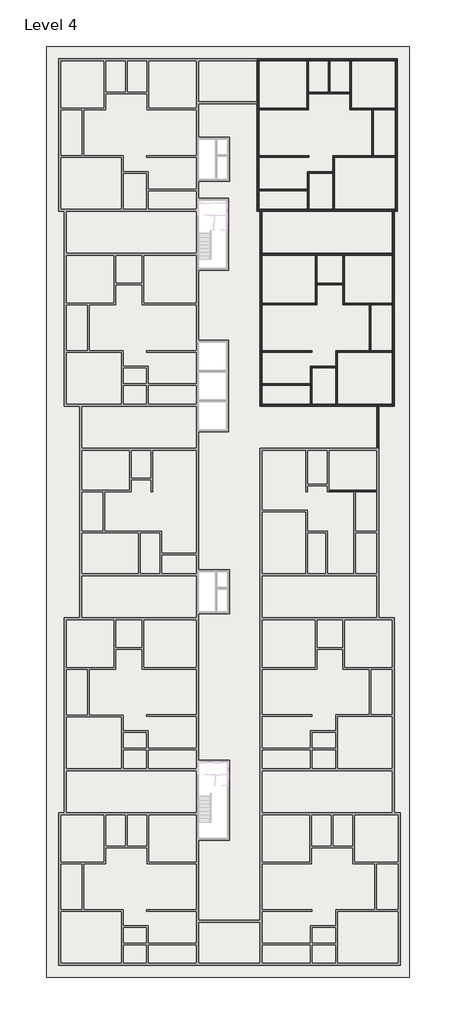
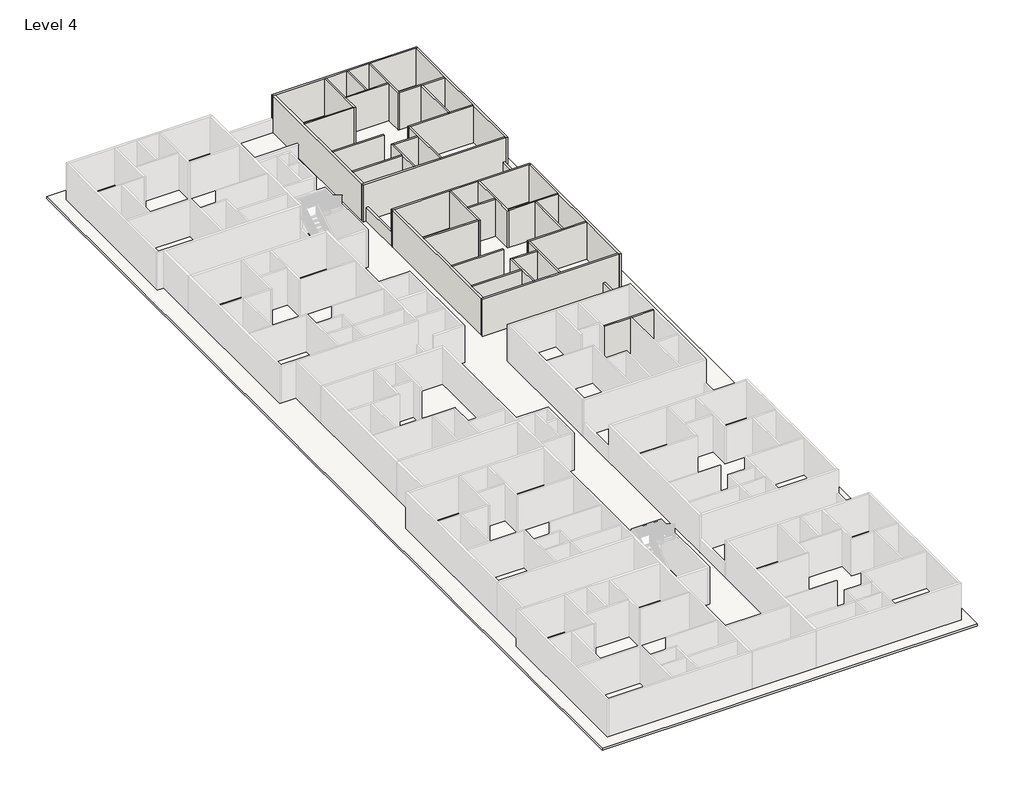
# One storey, part 4 of 8: 37 walls, 1 roof, 1 slab.
"""IFC4 building model written with IfcOpenShell, lengths in millimetres."""

from ifc_helpers import new_model, si_unit, frame, origin, place, context, project, spatial, polyline, outline, extrude, faceted_brep, element, save

model = new_model("IFC4")

# Units and contexts
model_context = context("Model", 3, world=origin())
ifc_project = project(units=[si_unit("LENGTHUNIT", "METRE", prefix="MILLI")], contexts=[model_context])

# Site, building, storey
site = spatial("IfcSite", under=ifc_project)
building = spatial("IfcBuilding", under=site)
storey = spatial("IfcBuildingStorey", under=building, Name="Level 4", Elevation=34378.6172466)

# Roof
placement = place(None, origin())
element("IfcRoof", 1, ObjectType="SLAB", at=placement, inside=storey, context=model_context, shape_type="SweptSolid", body=[
    extrude(outline(polyline([(-15237.9415084, -35021.5344126), (-15237.9415084, 36097.9216096), (12498.9443719, 36097.9216096), (12498.9443719, -35021.5344126), (-15237.9415084, -35021.5344126)]), holes=[polyline([(-3617.4415084, 29152.4900967), (-3617.4415084, 25799.6900967), (-1255.2415084, 25799.6900967), (-1255.2415084, 29152.4900967), (-3617.4415084, 29152.4900967)]), polyline([(-3617.4415084, 24490.1216096), (-3617.4415084, 19003.7216096), (-1331.4415084, 19003.7216096), (-1331.4415084, 24490.1216096), (-3617.4415084, 24490.1216096)]), polyline([(-3617.4415084, 13669.6303368), (-3617.4415084, 6659.2303368), (-1331.4415084, 6659.2303368), (-1331.4415084, 13669.6303368), (-3617.4415084, 13669.6303368)]), polyline([(-3617.4415084, -3882.2751812), (-3617.4415084, -7235.0751812), (-1255.2415084, -7235.0751812), (-1255.2415084, -3882.2751812), (-3617.4415084, -3882.2751812)]), polyline([(-3617.4415084, -18429.9851539), (-3617.4415084, -24525.9851539), (-1229.8415084, -24525.9851539), (-1229.8415084, -18429.9851539), (-3617.4415084, -18429.9851539)])]), frame((0.0, 0.0, 34378.6172466), z_axis=(0.0, 0.0, 1.0), x_axis=(1.0, 0.0, 0.0)), (0.0, 0.0, 1.0), 152.4),
])

# Slab
element("IfcSlab", 2, ObjectType="FLOOR", at=placement, inside=storey, context=model_context, shape_type="SweptSolid", body=[
    extrude(outline(polyline([(-14323.5415084, 35183.5216096), (11584.5443719, 35183.5216096), (11584.5443719, 23499.5216096), (11360.9214687, 23499.5216096), (11360.9214687, 8615.1216096), (10173.4714687, 8615.1216096), (10173.4714687, -7538.7344126), (11360.9214687, -7538.7344126), (11360.9214687, -22423.1344126), (11813.0584916, -22423.1344126), (11813.0584916, -34107.1344126), (11584.5443719, -34107.1344126), (-14323.5415084, -34107.1344126), (-14323.5415084, 35183.5216096)]), holes=[polyline([(-3617.4415084, 29152.4900967), (-3617.4415084, 25799.6900967), (-1255.2415084, 25799.6900967), (-1255.2415084, 29152.4900967), (-3617.4415084, 29152.4900967)]), polyline([(-3617.4415084, 24490.1216096), (-3617.4415084, 19003.7216096), (-1331.4415084, 19003.7216096), (-1331.4415084, 24490.1216096), (-3617.4415084, 24490.1216096)]), polyline([(-3617.4415084, 13669.6303368), (-3617.4415084, 6659.2303368), (-1331.4415084, 6659.2303368), (-1331.4415084, 13669.6303368), (-3617.4415084, 13669.6303368)]), polyline([(-3617.4415084, -3882.2751812), (-3617.4415084, -7235.0751812), (-1255.2415084, -7235.0751812), (-1255.2415084, -3882.2751812), (-3617.4415084, -3882.2751812)]), polyline([(-3617.4415084, -18429.9851539), (-3617.4415084, -24525.9851539), (-1229.8415084, -24525.9851539), (-1229.8415084, -18429.9851539), (-3617.4415084, -18429.9851539)])]), frame((0.0, 0.0, 33769.0172466), z_axis=(0.0, 0.0, 1.0), x_axis=(1.0, 0.0, 0.0)), (0.0, 0.0, 1.0), 609.6),
])

# Walls
element("IfcWall", 3, ObjectType="4.5\"", at=placement, inside=storey, context=model_context, shape_type="Brep", body=[
    faceted_brep([(6363.4714687, 2100.0216096, 34378.6172466), (8282.4584916, 2100.0216096, 34378.6172466), (8396.7584916, 2100.0216096, 34378.6172466), (10021.0714687, 2100.0216096, 34378.6172466), (10021.0714687, 2100.0216096, 37426.6172466), (8396.7584916, 2100.0216096, 37426.6172466), (8282.4584916, 2100.0216096, 37426.6172466), (6363.4714687, 2100.0216096, 37426.6172466), (6363.4714687, 2214.3216096, 34378.6172466), (6363.4714687, 2214.3216096, 37426.6172466), (10021.0714687, 2214.3216096, 37426.6172466), (10021.0714687, 2214.3216096, 34378.6172466)], [[[0, 1, 2, 3, 4, 5, 6, 7]], [[8, 9, 10, 11]], [[3, 2, 1, 0, 8, 11]], [[0, 7, 9, 8]], [[4, 3, 11, 10]], [[7, 6, 5, 4, 10, 9]]]),
])
element("IfcWall", 4, ObjectType="4.5\"", at=placement, inside=storey, context=model_context, shape_type="Brep", body=[
    faceted_brep([(5315.7214687, 20146.7216096, 34378.6172466), (5315.7214687, 16489.1216096, 34378.6172466), (5315.7214687, 16374.8216096, 34378.6172466), (5315.7214687, 16374.8216096, 37426.6172466), (5315.7214687, 16489.1216096, 37426.6172466), (5315.7214687, 20146.7216096, 37426.6172466), (5430.0214687, 20146.7216096, 34378.6172466), (5430.0214687, 20146.7216096, 37426.6172466), (5430.0214687, 18013.1216096, 37426.6172466), (5430.0214687, 17898.8216096, 37426.6172466), (5430.0214687, 16374.8216096, 37426.6172466), (5430.0214687, 16374.8216096, 34378.6172466), (5430.0214687, 17898.8216096, 34378.6172466), (5430.0214687, 18013.1216096, 34378.6172466)], [[[0, 1, 2, 3, 4, 5]], [[6, 7, 8, 9, 10, 11, 12, 13]], [[2, 1, 0, 6, 13, 12, 11]], [[0, 5, 7, 6]], [[3, 2, 11, 10]], [[5, 4, 3, 10, 9, 8, 7]]]),
])
element("IfcWall", 5, ObjectType="4.5\"", at=placement, inside=storey, context=model_context, shape_type="SweptSolid", body=[
    extrude(outline(polyline([(1259.3584916, 16489.1216096), (5315.7214687, 16489.1216096), (5315.7214687, 16374.8216096), (1259.3584916, 16374.8216096), (1259.3584916, 16489.1216096)])), frame((0.0, 0.0, 34378.6172466), z_axis=(0.0, 0.0, 1.0), x_axis=(1.0, 0.0, 0.0)), (0.0, 0.0, 1.0), 3048.0),
])
element("IfcWall", 6, ObjectType="4.5\"", at=placement, inside=storey, context=model_context, shape_type="SweptSolid", body=[
    extrude(outline(polyline([(7436.6214687, 17898.8216096), (5430.0214687, 17898.8216096), (5430.0214687, 18013.1216096), (7436.6214687, 18013.1216096), (7436.6214687, 17898.8216096)])), frame((0.0, 0.0, 34378.6172466), z_axis=(0.0, 0.0, 1.0), x_axis=(1.0, 0.0, 0.0)), (0.0, 0.0, 1.0), 3048.0),
])
element("IfcWall", 7, ObjectType="4.5\"", at=placement, inside=storey, context=model_context, shape_type="Brep", body=[
    faceted_brep([(7436.6214687, 20146.7216096, 34378.6172466), (7436.6214687, 18013.1216096, 34378.6172466), (7436.6214687, 17898.8216096, 34378.6172466), (7436.6214687, 16374.8216096, 34378.6172466), (7436.6214687, 16374.8216096, 37426.6172466), (7436.6214687, 17898.8216096, 37426.6172466), (7436.6214687, 18013.1216096, 37426.6172466), (7436.6214687, 20146.7216096, 37426.6172466), (7550.9214687, 20146.7216096, 34378.6172466), (7550.9214687, 20146.7216096, 37426.6172466), (7550.9214687, 16489.1216096, 37426.6172466), (7550.9214687, 16374.8216096, 37426.6172466), (7550.9214687, 16374.8216096, 34378.6172466), (7550.9214687, 16489.1216096, 34378.6172466)], [[[0, 1, 2, 3, 4, 5, 6, 7]], [[8, 9, 10, 11, 12, 13]], [[3, 2, 1, 0, 8, 13, 12]], [[0, 7, 9, 8]], [[4, 3, 12, 11]], [[7, 6, 5, 4, 11, 10, 9]]]),
])
element("IfcWall", 8, ObjectType="4.5\"", at=placement, inside=storey, context=model_context, shape_type="Brep", body=[
    faceted_brep([(7550.9214687, 16374.8216096, 34378.6172466), (9469.9084916, 16374.8216096, 34378.6172466), (9584.2084916, 16374.8216096, 34378.6172466), (11208.5214687, 16374.8216096, 34378.6172466), (11208.5214687, 16374.8216096, 37426.6172466), (9584.2084916, 16374.8216096, 37426.6172466), (9469.9084916, 16374.8216096, 37426.6172466), (7550.9214687, 16374.8216096, 37426.6172466), (7550.9214687, 16489.1216096, 34378.6172466), (7550.9214687, 16489.1216096, 37426.6172466), (11208.5214687, 16489.1216096, 37426.6172466), (11208.5214687, 16489.1216096, 34378.6172466)], [[[0, 1, 2, 3, 4, 5, 6, 7]], [[8, 9, 10, 11]], [[3, 2, 1, 0, 8, 11]], [[0, 7, 9, 8]], [[4, 3, 11, 10]], [[7, 6, 5, 4, 10, 9]]]),
])
element("IfcWall", 9, ObjectType="4.5\"", at=placement, inside=storey, context=model_context, shape_type="SweptSolid", body=[
    extrude(outline(polyline([(9469.9084916, 12869.6216096), (9469.9084916, 16374.8216096), (9584.2084916, 16374.8216096), (9584.2084916, 12869.6216096), (9469.9084916, 12869.6216096)])), frame((0.0, 0.0, 34378.6172466), z_axis=(0.0, 0.0, 1.0), x_axis=(1.0, 0.0, 0.0)), (0.0, 0.0, 1.0), 3048.0),
])
element("IfcWall", 10, ObjectType="4.5\"", at=placement, inside=storey, context=model_context, shape_type="Brep", body=[
    faceted_brep([(11208.5214687, 12869.6216096, 34378.6172466), (9584.2084916, 12869.6216096, 34378.6172466), (9469.9084916, 12869.6216096, 34378.6172466), (6885.4584916, 12869.6216096, 34378.6172466), (6885.4584916, 12869.6216096, 37426.6172466), (9469.9084916, 12869.6216096, 37426.6172466), (9584.2084916, 12869.6216096, 37426.6172466), (11208.5214687, 12869.6216096, 37426.6172466), (11208.5214687, 12755.3216096, 34378.6172466), (11208.5214687, 12755.3216096, 37426.6172466), (6999.7584916, 12755.3216096, 37426.6172466), (6885.4584916, 12755.3216096, 37426.6172466), (6885.4584916, 12755.3216096, 34378.6172466), (6999.7584916, 12755.3216096, 34378.6172466)], [[[0, 1, 2, 3, 4, 5, 6, 7]], [[8, 9, 10, 11, 12, 13]], [[3, 2, 1, 0, 8, 13, 12]], [[0, 7, 9, 8]], [[4, 3, 12, 11]], [[7, 6, 5, 4, 11, 10, 9]]]),
])
element("IfcWall", 11, ObjectType="4.5\"", at=placement, inside=storey, context=model_context, shape_type="Brep", body=[
    faceted_brep([(6885.4584916, 12755.3216096, 34378.6172466), (6885.4584916, 11663.1216096, 34378.6172466), (6885.4584916, 11548.8216096, 34378.6172466), (6885.4584916, 8767.5216096, 34378.6172466), (6885.4584916, 8767.5216096, 37426.6172466), (6885.4584916, 11548.8216096, 37426.6172466), (6885.4584916, 11663.1216096, 37426.6172466), (6885.4584916, 12755.3216096, 37426.6172466), (6999.7584916, 12755.3216096, 34378.6172466), (6999.7584916, 12755.3216096, 37426.6172466), (6999.7584916, 8767.5216096, 37426.6172466), (6999.7584916, 8767.5216096, 34378.6172466)], [[[0, 1, 2, 3, 4, 5, 6, 7]], [[8, 9, 10, 11]], [[3, 2, 1, 0, 8, 11]], [[0, 7, 9, 8]], [[4, 3, 11, 10]], [[7, 6, 5, 4, 10, 9]]]),
])
element("IfcWall", 12, ObjectType="4.5\"", at=placement, inside=storey, context=model_context, shape_type="Brep", body=[
    faceted_brep([(5056.6584916, 8767.5216096, 34378.6172466), (5056.6584916, 11548.8216096, 34378.6172466), (5056.6584916, 11663.1216096, 34378.6172466), (5056.6584916, 11663.1216096, 37426.6172466), (5056.6584916, 11548.8216096, 37426.6172466), (5056.6584916, 8767.5216096, 37426.6172466), (4942.3584916, 8767.5216096, 34378.6172466), (4942.3584916, 8767.5216096, 37426.6172466), (4942.3584916, 10215.3216096, 37426.6172466), (4942.3584916, 10329.6216096, 37426.6172466), (4942.3584916, 11663.1216096, 37426.6172466), (4942.3584916, 11663.1216096, 34378.6172466), (4942.3584916, 10329.6216096, 34378.6172466), (4942.3584916, 10215.3216096, 34378.6172466)], [[[0, 1, 2, 3, 4, 5]], [[6, 7, 8, 9, 10, 11, 12, 13]], [[2, 1, 0, 6, 13, 12, 11]], [[0, 5, 7, 6]], [[3, 2, 11, 10]], [[5, 4, 3, 10, 9, 8, 7]]]),
])
element("IfcWall", 13, ObjectType="4.5\"", at=placement, inside=storey, context=model_context, shape_type="SweptSolid", body=[
    extrude(outline(polyline([(6885.4584916, 11548.8216096), (5056.6584916, 11548.8216096), (5056.6584916, 11663.1216096), (6885.4584916, 11663.1216096), (6885.4584916, 11548.8216096)])), frame((0.0, 0.0, 34378.6172466), z_axis=(0.0, 0.0, 1.0), x_axis=(1.0, 0.0, 0.0)), (0.0, 0.0, 1.0), 3048.0),
])
element("IfcWall", 14, ObjectType="4.5\"", at=placement, inside=storey, context=model_context, shape_type="SweptSolid", body=[
    extrude(outline(polyline([(4942.3584916, 10215.3216096), (1259.3584916, 10215.3216096), (1259.3584916, 10329.6216096), (4942.3584916, 10329.6216096), (4942.3584916, 10215.3216096)])), frame((0.0, 0.0, 34378.6172466), z_axis=(0.0, 0.0, 1.0), x_axis=(1.0, 0.0, 0.0)), (0.0, 0.0, 1.0), 3048.0),
])
element("IfcWall", 15, ObjectType="4.5\"", at=placement, inside=storey, context=model_context, shape_type="SweptSolid", body=[
    extrude(outline(polyline([(5056.6584916, 12755.3216096), (1259.3584916, 12755.3216096), (1259.3584916, 12869.6216096), (5056.6584916, 12869.6216096), (5056.6584916, 12755.3216096)])), frame((0.0, 0.0, 34378.6172466), z_axis=(0.0, 0.0, 1.0), x_axis=(1.0, 0.0, 0.0)), (0.0, 0.0, 1.0), 3048.0),
])
element("IfcWall", 16, ObjectType="4.5\"", at=placement, inside=storey, context=model_context, shape_type="Brep", body=[
    faceted_brep([(4688.4443719, 35031.1216096, 34378.6172466), (4688.4443719, 31373.5216096, 34378.6172466), (4688.4443719, 31259.2216096, 34378.6172466), (4688.4443719, 31259.2216096, 37426.6172466), (4688.4443719, 31373.5216096, 37426.6172466), (4688.4443719, 35031.1216096, 37426.6172466), (4802.7443719, 35031.1216096, 34378.6172466), (4802.7443719, 35031.1216096, 37426.6172466), (4802.7443719, 32592.7216096, 37426.6172466), (4802.7443719, 32478.4216096, 37426.6172466), (4802.7443719, 31259.2216096, 37426.6172466), (4802.7443719, 31259.2216096, 34378.6172466), (4802.7443719, 32478.4216096, 34378.6172466), (4802.7443719, 32592.7216096, 34378.6172466)], [[[0, 1, 2, 3, 4, 5]], [[6, 7, 8, 9, 10, 11, 12, 13]], [[2, 1, 0, 6, 13, 12, 11]], [[0, 5, 7, 6]], [[3, 2, 11, 10]], [[5, 4, 3, 10, 9, 8, 7]]]),
])
element("IfcWall", 17, ObjectType="4.5\"", at=placement, inside=storey, context=model_context, shape_type="SweptSolid", body=[
    extrude(outline(polyline([(1030.8443719, 31373.5216096), (4688.4443719, 31373.5216096), (4688.4443719, 31259.2216096), (1030.8443719, 31259.2216096), (1030.8443719, 31373.5216096)])), frame((0.0, 0.0, 34378.6172466), z_axis=(0.0, 0.0, 1.0), x_axis=(1.0, 0.0, 0.0)), (0.0, 0.0, 1.0), 3048.0),
])
element("IfcWall", 18, ObjectType="4.5\"", at=placement, inside=storey, context=model_context, shape_type="Brep", body=[
    faceted_brep([(4802.7443719, 32478.4216096, 34378.6172466), (7965.0443719, 32478.4216096, 34378.6172466), (7965.0443719, 32478.4216096, 37426.6172466), (4802.7443719, 32478.4216096, 37426.6172466), (4802.7443719, 32592.7216096, 34378.6172466), (4802.7443719, 32592.7216096, 37426.6172466), (6326.7443719, 32592.7216096, 37426.6172466), (6441.0443719, 32592.7216096, 37426.6172466), (7965.0443719, 32592.7216096, 37426.6172466), (7965.0443719, 32592.7216096, 34378.6172466), (6441.0443719, 32592.7216096, 34378.6172466), (6326.7443719, 32592.7216096, 34378.6172466)], [[[0, 1, 2, 3]], [[4, 5, 6, 7, 8, 9, 10, 11]], [[1, 0, 4, 11, 10, 9]], [[0, 3, 5, 4]], [[2, 1, 9, 8]], [[3, 2, 8, 7, 6, 5]]]),
])
element("IfcWall", 19, ObjectType="4.5\"", at=placement, inside=storey, context=model_context, shape_type="SweptSolid", body=[
    extrude(outline(polyline([(6326.7443719, 32592.7216096), (6326.7443719, 35031.1216096), (6441.0443719, 35031.1216096), (6441.0443719, 32592.7216096), (6326.7443719, 32592.7216096)])), frame((0.0, 0.0, 34378.6172466), z_axis=(0.0, 0.0, 1.0), x_axis=(1.0, 0.0, 0.0)), (0.0, 0.0, 1.0), 3048.0),
])
element("IfcWall", 20, ObjectType="4.5\"", at=placement, inside=storey, context=model_context, shape_type="Brep", body=[
    faceted_brep([(7965.0443719, 35031.1216096, 34378.6172466), (7965.0443719, 32592.7216096, 34378.6172466), (7965.0443719, 32478.4216096, 34378.6172466), (7965.0443719, 31259.2216096, 34378.6172466), (7965.0443719, 31259.2216096, 37426.6172466), (7965.0443719, 32478.4216096, 37426.6172466), (7965.0443719, 32592.7216096, 37426.6172466), (7965.0443719, 35031.1216096, 37426.6172466), (8079.3443719, 35031.1216096, 34378.6172466), (8079.3443719, 35031.1216096, 37426.6172466), (8079.3443719, 31373.5216096, 37426.6172466), (8079.3443719, 31259.2216096, 37426.6172466), (8079.3443719, 31259.2216096, 34378.6172466), (8079.3443719, 31373.5216096, 34378.6172466)], [[[0, 1, 2, 3, 4, 5, 6, 7]], [[8, 9, 10, 11, 12, 13]], [[3, 2, 1, 0, 8, 13, 12]], [[0, 7, 9, 8]], [[4, 3, 12, 11]], [[7, 6, 5, 4, 11, 10, 9]]]),
])
element("IfcWall", 21, ObjectType="4.5\"", at=placement, inside=storey, context=model_context, shape_type="Brep", body=[
    faceted_brep([(8079.3443719, 31259.2216096, 34378.6172466), (9641.4443719, 31259.2216096, 34378.6172466), (9755.7443719, 31259.2216096, 34378.6172466), (11432.1443719, 31259.2216096, 34378.6172466), (11432.1443719, 31259.2216096, 37426.6172466), (9755.7443719, 31259.2216096, 37426.6172466), (9641.4443719, 31259.2216096, 37426.6172466), (8079.3443719, 31259.2216096, 37426.6172466), (8079.3443719, 31373.5216096, 34378.6172466), (8079.3443719, 31373.5216096, 37426.6172466), (11432.1443719, 31373.5216096, 37426.6172466), (11432.1443719, 31373.5216096, 34378.6172466)], [[[0, 1, 2, 3, 4, 5, 6, 7]], [[8, 9, 10, 11]], [[3, 2, 1, 0, 8, 11]], [[0, 7, 9, 8]], [[4, 3, 11, 10]], [[7, 6, 5, 4, 10, 9]]]),
])
element("IfcWall", 22, ObjectType="4.5\"", at=placement, inside=storey, context=model_context, shape_type="SweptSolid", body=[
    extrude(outline(polyline([(9641.4443719, 27754.0216096), (9641.4443719, 31259.2216096), (9755.7443719, 31259.2216096), (9755.7443719, 27754.0216096), (9641.4443719, 27754.0216096)])), frame((0.0, 0.0, 34378.6172466), z_axis=(0.0, 0.0, 1.0), x_axis=(1.0, 0.0, 0.0)), (0.0, 0.0, 1.0), 3048.0),
])
element("IfcWall", 23, ObjectType="4.5\"", at=placement, inside=storey, context=model_context, shape_type="Brep", body=[
    faceted_brep([(11432.1443719, 27754.0216096, 34378.6172466), (9755.7443719, 27754.0216096, 34378.6172466), (9641.4443719, 27754.0216096, 34378.6172466), (6656.9443719, 27754.0216096, 34378.6172466), (6656.9443719, 27754.0216096, 37426.6172466), (9641.4443719, 27754.0216096, 37426.6172466), (9755.7443719, 27754.0216096, 37426.6172466), (11432.1443719, 27754.0216096, 37426.6172466), (11432.1443719, 27639.7216096, 34378.6172466), (11432.1443719, 27639.7216096, 37426.6172466), (6771.2443719, 27639.7216096, 37426.6172466), (6656.9443719, 27639.7216096, 37426.6172466), (6656.9443719, 27639.7216096, 34378.6172466), (6771.2443719, 27639.7216096, 34378.6172466)], [[[0, 1, 2, 3, 4, 5, 6, 7]], [[8, 9, 10, 11, 12, 13]], [[3, 2, 1, 0, 8, 13, 12]], [[0, 7, 9, 8]], [[4, 3, 12, 11]], [[7, 6, 5, 4, 11, 10, 9]]]),
])
element("IfcWall", 24, ObjectType="4.5\"", at=placement, inside=storey, context=model_context, shape_type="Brep", body=[
    faceted_brep([(6656.9443719, 27639.7216096, 34378.6172466), (6656.9443719, 26547.5216096, 34378.6172466), (6656.9443719, 26433.2216096, 34378.6172466), (6656.9443719, 23651.9216096, 34378.6172466), (6656.9443719, 23651.9216096, 37426.6172466), (6656.9443719, 26433.2216096, 37426.6172466), (6656.9443719, 26547.5216096, 37426.6172466), (6656.9443719, 27639.7216096, 37426.6172466), (6771.2443719, 27639.7216096, 34378.6172466), (6771.2443719, 27639.7216096, 37426.6172466), (6771.2443719, 23651.9216096, 37426.6172466), (6771.2443719, 23651.9216096, 34378.6172466)], [[[0, 1, 2, 3, 4, 5, 6, 7]], [[8, 9, 10, 11]], [[3, 2, 1, 0, 8, 11]], [[0, 7, 9, 8]], [[4, 3, 11, 10]], [[7, 6, 5, 4, 10, 9]]]),
])
element("IfcWall", 25, ObjectType="4.5\"", at=placement, inside=storey, context=model_context, shape_type="SweptSolid", body=[
    extrude(outline(polyline([(4713.8443719, 25099.7216096), (1030.8443719, 25099.7216096), (1030.8443719, 25214.0216096), (4713.8443719, 25214.0216096), (4713.8443719, 25099.7216096)])), frame((0.0, 0.0, 34378.6172466), z_axis=(0.0, 0.0, 1.0), x_axis=(1.0, 0.0, 0.0)), (0.0, 0.0, 1.0), 3048.0),
])
element("IfcWall", 26, ObjectType="4.5\"", at=placement, inside=storey, context=model_context, shape_type="Brep", body=[
    faceted_brep([(4828.1443719, 23651.9216096, 34378.6172466), (4828.1443719, 26433.2216096, 34378.6172466), (4828.1443719, 26547.5216096, 34378.6172466), (4828.1443719, 26547.5216096, 37426.6172466), (4828.1443719, 26433.2216096, 37426.6172466), (4828.1443719, 23651.9216096, 37426.6172466), (4713.8443719, 23651.9216096, 34378.6172466), (4713.8443719, 23651.9216096, 37426.6172466), (4713.8443719, 25099.7216096, 37426.6172466), (4713.8443719, 25214.0216096, 37426.6172466), (4713.8443719, 26547.5216096, 37426.6172466), (4713.8443719, 26547.5216096, 34378.6172466), (4713.8443719, 25214.0216096, 34378.6172466), (4713.8443719, 25099.7216096, 34378.6172466)], [[[0, 1, 2, 3, 4, 5]], [[6, 7, 8, 9, 10, 11, 12, 13]], [[2, 1, 0, 6, 13, 12, 11]], [[0, 5, 7, 6]], [[3, 2, 11, 10]], [[5, 4, 3, 10, 9, 8, 7]]]),
])
element("IfcWall", 27, ObjectType="4.5\"", at=placement, inside=storey, context=model_context, shape_type="SweptSolid", body=[
    extrude(outline(polyline([(6656.9443719, 26433.2216096), (4828.1443719, 26433.2216096), (4828.1443719, 26547.5216096), (6656.9443719, 26547.5216096), (6656.9443719, 26433.2216096)])), frame((0.0, 0.0, 34378.6172466), z_axis=(0.0, 0.0, 1.0), x_axis=(1.0, 0.0, 0.0)), (0.0, 0.0, 1.0), 3048.0),
])
element("IfcWall", 28, ObjectType="4.5\"", at=placement, inside=storey, context=model_context, shape_type="SweptSolid", body=[
    extrude(outline(polyline([(4828.1443719, 27639.7216096), (1030.8443719, 27639.7216096), (1030.8443719, 27754.0216096), (4828.1443719, 27754.0216096), (4828.1443719, 27639.7216096)])), frame((0.0, 0.0, 34378.6172466), z_axis=(0.0, 0.0, 1.0), x_axis=(1.0, 0.0, 0.0)), (0.0, 0.0, 1.0), 3048.0),
])
element("IfcWall", 29, ObjectType="6\"", at=placement, inside=storey, context=model_context, shape_type="Brep", body=[
    faceted_brep([(1106.9584916, 20146.7216096, 37426.6172466), (1106.9584916, 20146.7216096, 34378.6172466), (1259.3584916, 20146.7216096, 34378.6172466), (5315.7214687, 20146.7216096, 34378.6172466), (5430.0214687, 20146.7216096, 34378.6172466), (7436.6214687, 20146.7216096, 34378.6172466), (7550.9214687, 20146.7216096, 34378.6172466), (11208.5214687, 20146.7216096, 34378.6172466), (11360.9214687, 20146.7216096, 34378.6172466), (11360.9214687, 20146.7216096, 37426.6172466), (11208.5214687, 20146.7216096, 37426.6172466), (7550.9214687, 20146.7216096, 37426.6172466), (7436.6214687, 20146.7216096, 37426.6172466), (5430.0214687, 20146.7216096, 37426.6172466), (5315.7214687, 20146.7216096, 37426.6172466), (1259.3584916, 20146.7216096, 37426.6172466), (1106.9584916, 20299.1216096, 34378.6172466), (1106.9584916, 20299.1216096, 35597.8172466), (1106.9584916, 20299.1216096, 37426.6172466), (11360.9214687, 20299.1216096, 37426.6172466), (11360.9214687, 20299.1216096, 35597.8172466), (11360.9214687, 20299.1216096, 34378.6172466), (11208.5214687, 20299.1216096, 34378.6172466), (1259.3584916, 20299.1216096, 34378.6172466)], [[[0, 1, 2, 3, 4, 5, 6, 7, 8, 9, 10, 11, 12, 13, 14, 15]], [[16, 17, 18, 19, 20, 21, 22, 23]], [[8, 7, 6, 5, 4, 3, 2, 1, 16, 23, 22, 21]], [[0, 18, 17, 16, 1]], [[8, 21, 20, 19, 9]], [[0, 15, 14, 13, 12, 11, 10, 9, 19, 18]]]),
])
element("IfcWall", 30, ObjectType="6\"", at=placement, inside=storey, context=model_context, shape_type="Brep", body=[
    faceted_brep([(11208.5214687, 20146.7216096, 37426.6172466), (11208.5214687, 20146.7216096, 34378.6172466), (11208.5214687, 16489.1216096, 34378.6172466), (11208.5214687, 16374.8216096, 34378.6172466), (11208.5214687, 12869.6216096, 34378.6172466), (11208.5214687, 12755.3216096, 34378.6172466), (11208.5214687, 8767.5216096, 34378.6172466), (11208.5214687, 8615.1216096, 34378.6172466), (11208.5214687, 8615.1216096, 37426.6172466), (11208.5214687, 8767.5216096, 37426.6172466), (11208.5214687, 12755.3216096, 37426.6172466), (11208.5214687, 12869.6216096, 37426.6172466), (11208.5214687, 16374.8216096, 37426.6172466), (11208.5214687, 16489.1216096, 37426.6172466), (11360.9214687, 20146.7216096, 34378.6172466), (11360.9214687, 20146.7216096, 37426.6172466), (11360.9214687, 8615.1216096, 37426.6172466), (11360.9214687, 8615.1216096, 34378.6172466)], [[[0, 1, 2, 3, 4, 5, 6, 7, 8, 9, 10, 11, 12, 13]], [[14, 15, 16, 17]], [[7, 6, 5, 4, 3, 2, 1, 14, 17]], [[8, 7, 17, 16]], [[0, 15, 14, 1]], [[0, 13, 12, 11, 10, 9, 8, 16, 15]]]),
])
element("IfcWall", 31, ObjectType="6\"", at=placement, inside=storey, context=model_context, shape_type="Brep", body=[
    faceted_brep([(11208.5214687, 8767.5216096, 34378.6172466), (6999.7584916, 8767.5216096, 34378.6172466), (6885.4584916, 8767.5216096, 34378.6172466), (5056.6584916, 8767.5216096, 34378.6172466), (4942.3584916, 8767.5216096, 34378.6172466), (1259.3584916, 8767.5216096, 34378.6172466), (1106.9584916, 8767.5216096, 34378.6172466), (1106.9584916, 8767.5216096, 37426.6172466), (1259.3584916, 8767.5216096, 37426.6172466), (4942.3584916, 8767.5216096, 37426.6172466), (5056.6584916, 8767.5216096, 37426.6172466), (6885.4584916, 8767.5216096, 37426.6172466), (6999.7584916, 8767.5216096, 37426.6172466), (11208.5214687, 8767.5216096, 37426.6172466), (11208.5214687, 8615.1216096, 34378.6172466), (11208.5214687, 8615.1216096, 37426.6172466), (1106.9584916, 8615.1216096, 37426.6172466), (1106.9584916, 8615.1216096, 34378.6172466), (10021.0714687, 8615.1216096, 34378.6172466), (10173.4714687, 8615.1216096, 34378.6172466)], [[[0, 1, 2, 3, 4, 5, 6, 7, 8, 9, 10, 11, 12, 13]], [[14, 15, 16, 17, 18, 19]], [[6, 5, 4, 3, 2, 1, 0, 14, 19, 18, 17]], [[0, 13, 15, 14]], [[7, 6, 17, 16]], [[13, 12, 11, 10, 9, 8, 7, 16, 15]]]),
])
element("IfcWall", 32, ObjectType="6\"", at=placement, inside=storey, context=model_context, shape_type="Brep", body=[
    faceted_brep([(1259.3584916, 8767.5216096, 34378.6172466), (1259.3584916, 10215.3216096, 34378.6172466), (1259.3584916, 10329.6216096, 34378.6172466), (1259.3584916, 12755.3216096, 34378.6172466), (1259.3584916, 12869.6216096, 34378.6172466), (1259.3584916, 16374.8216096, 34378.6172466), (1259.3584916, 16489.1216096, 34378.6172466), (1259.3584916, 20146.7216096, 34378.6172466), (1259.3584916, 20146.7216096, 37426.6172466), (1259.3584916, 16489.1216096, 37426.6172466), (1259.3584916, 16374.8216096, 37426.6172466), (1259.3584916, 12869.6216096, 37426.6172466), (1259.3584916, 12755.3216096, 37426.6172466), (1259.3584916, 10329.6216096, 37426.6172466), (1259.3584916, 10215.3216096, 37426.6172466), (1259.3584916, 8767.5216096, 37426.6172466), (1106.9584916, 8767.5216096, 34378.6172466), (1106.9584916, 8767.5216096, 37426.6172466), (1106.9584916, 20146.7216096, 37426.6172466), (1106.9584916, 20146.7216096, 34378.6172466)], [[[0, 1, 2, 3, 4, 5, 6, 7, 8, 9, 10, 11, 12, 13, 14, 15]], [[16, 17, 18, 19]], [[7, 6, 5, 4, 3, 2, 1, 0, 16, 19]], [[0, 15, 17, 16]], [[7, 19, 18, 8]], [[15, 14, 13, 12, 11, 10, 9, 8, 18, 17]]]),
])
element("IfcWall", 33, ObjectType="6\"", at=placement, inside=storey, context=model_context, shape_type="Brep", body=[
    faceted_brep([(878.4443719, 35031.1216096, 37426.6172466), (878.4443719, 35031.1216096, 34378.6172466), (1030.8443719, 35031.1216096, 34378.6172466), (4688.4443719, 35031.1216096, 34378.6172466), (4802.7443719, 35031.1216096, 34378.6172466), (6326.7443719, 35031.1216096, 34378.6172466), (6441.0443719, 35031.1216096, 34378.6172466), (7965.0443719, 35031.1216096, 34378.6172466), (8079.3443719, 35031.1216096, 34378.6172466), (11432.1443719, 35031.1216096, 34378.6172466), (11584.5443719, 35031.1216096, 34378.6172466), (11584.5443719, 35031.1216096, 37426.6172466), (11432.1443719, 35031.1216096, 37426.6172466), (8079.3443719, 35031.1216096, 37426.6172466), (7965.0443719, 35031.1216096, 37426.6172466), (6441.0443719, 35031.1216096, 37426.6172466), (6326.7443719, 35031.1216096, 37426.6172466), (4802.7443719, 35031.1216096, 37426.6172466), (4688.4443719, 35031.1216096, 37426.6172466), (1030.8443719, 35031.1216096, 37426.6172466), (878.4443719, 35183.5216096, 34378.6172466), (878.4443719, 35183.5216096, 37426.6172466), (11584.5443719, 35183.5216096, 37426.6172466), (11584.5443719, 35183.5216096, 34378.6172466)], [[[0, 1, 2, 3, 4, 5, 6, 7, 8, 9, 10, 11, 12, 13, 14, 15, 16, 17, 18, 19]], [[20, 21, 22, 23]], [[10, 9, 8, 7, 6, 5, 4, 3, 2, 1, 20, 23]], [[11, 10, 23, 22]], [[0, 21, 20, 1]], [[0, 19, 18, 17, 16, 15, 14, 13, 12, 11, 22, 21]]]),
])
element("IfcWall", 34, ObjectType="6\"", at=placement, inside=storey, context=model_context, shape_type="Brep", body=[
    faceted_brep([(11432.1443719, 35031.1216096, 34378.6172466), (11432.1443719, 31373.5216096, 34378.6172466), (11432.1443719, 31259.2216096, 34378.6172466), (11432.1443719, 27754.0216096, 34378.6172466), (11432.1443719, 27639.7216096, 34378.6172466), (11432.1443719, 23651.9216096, 34378.6172466), (11432.1443719, 23499.5216096, 34378.6172466), (11432.1443719, 23499.5216096, 37426.6172466), (11432.1443719, 23651.9216096, 37426.6172466), (11432.1443719, 27639.7216096, 37426.6172466), (11432.1443719, 27754.0216096, 37426.6172466), (11432.1443719, 31259.2216096, 37426.6172466), (11432.1443719, 31373.5216096, 37426.6172466), (11432.1443719, 35031.1216096, 37426.6172466), (11584.5443719, 35031.1216096, 34378.6172466), (11584.5443719, 35031.1216096, 37426.6172466), (11584.5443719, 23499.5216096, 37426.6172466), (11584.5443719, 23499.5216096, 34378.6172466)], [[[0, 1, 2, 3, 4, 5, 6, 7, 8, 9, 10, 11, 12, 13]], [[14, 15, 16, 17]], [[6, 5, 4, 3, 2, 1, 0, 14, 17]], [[0, 13, 15, 14]], [[7, 6, 17, 16]], [[13, 12, 11, 10, 9, 8, 7, 16, 15]]]),
])
element("IfcWall", 35, ObjectType="6\"", at=placement, inside=storey, context=model_context, shape_type="Brep", body=[
    faceted_brep([(11432.1443719, 23651.9216096, 34378.6172466), (6771.2443719, 23651.9216096, 34378.6172466), (6656.9443719, 23651.9216096, 34378.6172466), (4828.1443719, 23651.9216096, 34378.6172466), (4713.8443719, 23651.9216096, 34378.6172466), (1030.8443719, 23651.9216096, 34378.6172466), (878.4443719, 23651.9216096, 34378.6172466), (878.4443719, 23651.9216096, 37426.6172466), (1030.8443719, 23651.9216096, 37426.6172466), (4713.8443719, 23651.9216096, 37426.6172466), (4828.1443719, 23651.9216096, 37426.6172466), (6656.9443719, 23651.9216096, 37426.6172466), (6771.2443719, 23651.9216096, 37426.6172466), (11432.1443719, 23651.9216096, 37426.6172466), (11432.1443719, 23499.5216096, 34378.6172466), (11432.1443719, 23499.5216096, 37426.6172466), (878.4443719, 23499.5216096, 37426.6172466), (878.4443719, 23499.5216096, 34378.6172466), (1106.9584916, 23499.5216096, 34378.6172466), (1259.3584916, 23499.5216096, 34378.6172466), (11208.5214687, 23499.5216096, 34378.6172466), (11360.9214687, 23499.5216096, 34378.6172466)], [[[0, 1, 2, 3, 4, 5, 6, 7, 8, 9, 10, 11, 12, 13]], [[14, 15, 16, 17, 18, 19, 20, 21]], [[6, 5, 4, 3, 2, 1, 0, 14, 21, 20, 19, 18, 17]], [[0, 13, 15, 14]], [[7, 6, 17, 16]], [[13, 12, 11, 10, 9, 8, 7, 16, 15]]]),
])
element("IfcWall", 36, ObjectType="6\"", at=placement, inside=storey, context=model_context, shape_type="Brep", body=[
    faceted_brep([(1030.8443719, 23651.9216096, 34378.6172466), (1030.8443719, 25099.7216096, 34378.6172466), (1030.8443719, 25214.0216096, 34378.6172466), (1030.8443719, 27639.7216096, 34378.6172466), (1030.8443719, 27754.0216096, 34378.6172466), (1030.8443719, 31259.2216096, 34378.6172466), (1030.8443719, 31373.5216096, 34378.6172466), (1030.8443719, 35031.1216096, 34378.6172466), (1030.8443719, 35031.1216096, 37426.6172466), (1030.8443719, 31373.5216096, 37426.6172466), (1030.8443719, 31259.2216096, 37426.6172466), (1030.8443719, 27754.0216096, 37426.6172466), (1030.8443719, 27639.7216096, 37426.6172466), (1030.8443719, 25214.0216096, 37426.6172466), (1030.8443719, 25099.7216096, 37426.6172466), (1030.8443719, 23651.9216096, 37426.6172466), (878.4443719, 23651.9216096, 34378.6172466), (878.4443719, 23651.9216096, 37426.6172466), (878.4443719, 35031.1216096, 37426.6172466), (878.4443719, 35031.1216096, 34378.6172466), (878.4443719, 31897.3197155, 34378.6172466), (878.4443719, 31744.9197155, 34378.6172466)], [[[0, 1, 2, 3, 4, 5, 6, 7, 8, 9, 10, 11, 12, 13, 14, 15]], [[16, 17, 18, 19, 20, 21]], [[7, 6, 5, 4, 3, 2, 1, 0, 16, 21, 20, 19]], [[0, 15, 17, 16]], [[7, 19, 18, 8]], [[15, 14, 13, 12, 11, 10, 9, 8, 18, 17]]]),
])
element("IfcWall", 37, ObjectType="6\" 2", at=placement, inside=storey, context=model_context, shape_type="SweptSolid", body=[
    extrude(outline(polyline([(1106.9584916, 20299.1216096), (1106.9584916, 23499.5216096), (1259.3584916, 23499.5216096), (1259.3584916, 20299.1216096), (1106.9584916, 20299.1216096)])), frame((0.0, 0.0, 34378.6172466), z_axis=(0.0, 0.0, 1.0), x_axis=(1.0, 0.0, 0.0)), (0.0, 0.0, 1.0), 1219.2),
])
element("IfcWall", 38, ObjectType="6\" 2", at=placement, inside=storey, context=model_context, shape_type="SweptSolid", body=[
    extrude(outline(polyline([(11208.5214687, 20299.1216096), (11208.5214687, 23499.5216096), (11360.9214687, 23499.5216096), (11360.9214687, 20299.1216096), (11208.5214687, 20299.1216096)])), frame((0.0, 0.0, 34378.6172466), z_axis=(0.0, 0.0, 1.0), x_axis=(1.0, 0.0, 0.0)), (0.0, 0.0, 1.0), 1219.2),
])
element("IfcWall", 39, ObjectType="6\" 2", at=placement, inside=storey, context=model_context, shape_type="SweptSolid", body=[
    extrude(outline(polyline([(10021.0714687, 5414.7216096), (10021.0714687, 8615.1216096), (10173.4714687, 8615.1216096), (10173.4714687, 5414.7216096), (10021.0714687, 5414.7216096)])), frame((0.0, 0.0, 34378.6172466), z_axis=(0.0, 0.0, 1.0), x_axis=(1.0, 0.0, 0.0)), (0.0, 0.0, 1.0), 1219.2),
])

save(model, "model.ifc")

# Revit data of these elements
# Type "SLAB"
#   Assembly Code = "B1020"
#   Layers, outside or top first: 0' - 6" "Damp-proofing" (function 1)
# Type "FLOOR"
#   Assembly Code = "B1010"
#   Function = 0
#   Layers, outside or top first: 2' - 0" "Tile, Porcelain, 4in" (function 1)
# Type "4.5\""
#   Assembly Code = "B2010"
#   Layers, outside or top first: 0' - 4 1/2" "WALLS" (function 1)
# Type "6\""
#   Assembly Code = "B2010"
#   Layers, outside or top first: 0' - 6" "WALLS" (function 1)
# Type "6\" 2"
#   Assembly Code = "B2010"
#   Layers, outside or top first: 0' - 6" "4'" (function 1)
# Element 1 (IfcRoof, "SLAB")
#   built-in parameter 1001705 = 113.291 (stored number, unit not read)
#   built-in parameter 1001710 = 33615
#   Phase Created = New Construction
#   Materials on its faces: "Damp-proofing"
# Element 2 (IfcSlab, "FLOOR")
#   built-in parameter 1001955 = 3.14159 (stored number, unit not read)
#   Height Offset From Level = 0' - 0"
#   Phase Created = New Construction
#   Materials on its faces: "Tile, Porcelain, 4in"
# Elements 3, 4, 5, 6, 7, 8, 9, 10, 11, 12, 13, 14, 15, 16, 17, 18, 19, 20, 21, 22, 23, 24, 25, 26, 27, 28 (IfcWall, "4.5\"")
#   Top Offset = 0' - 0"
#   Base Offset = 0' - 0"
#   Unconnected Height = 10' - 0"
#   wall height = 10' - 0"
#   Phase Created = New Construction
#   Base Constraint = Level 4
#   Materials on its faces: "WALLS"
# Elements 29, 30, 31, 32, 33, 34, 35, 36 (IfcWall, "6\"")
#   Top Offset = 0' - 0"
#   Base Offset = 0' - 0"
#   Unconnected Height = 10' - 0"
#   wall height = 10' - 0"
#   Phase Created = New Construction
#   Base Constraint = Level 4
#   Materials on its faces: "WALLS"
# Elements 37, 38, 39 (IfcWall, "6\" 2")
#   Top Offset = 0' - 0"
#   Base Offset = 0' - 0"
#   Unconnected Height = 4' - 0"
#   wall height = 4' - 0"
#   Phase Created = New Construction
#   Base Constraint = Level 4
#   Materials on its faces: "4'"
# Materials
#   "Damp-proofing": class "Generic", colour RGB 127 127 127, transparency 0, Description = "Damp-proofing", Cost = 0
#   "Tile, Porcelain, 4in": class "Generic", colour RGB 89 87 158, transparency 0, Description = "Porcelain tile, 4\", white", Cost = 0
#   "WALLS": class "Generic", colour RGB 120 120 120, transparency 0, Cost = 0
#   "4'": class "Generic", colour RGB 120 120 120, transparency 0, Cost = 0
